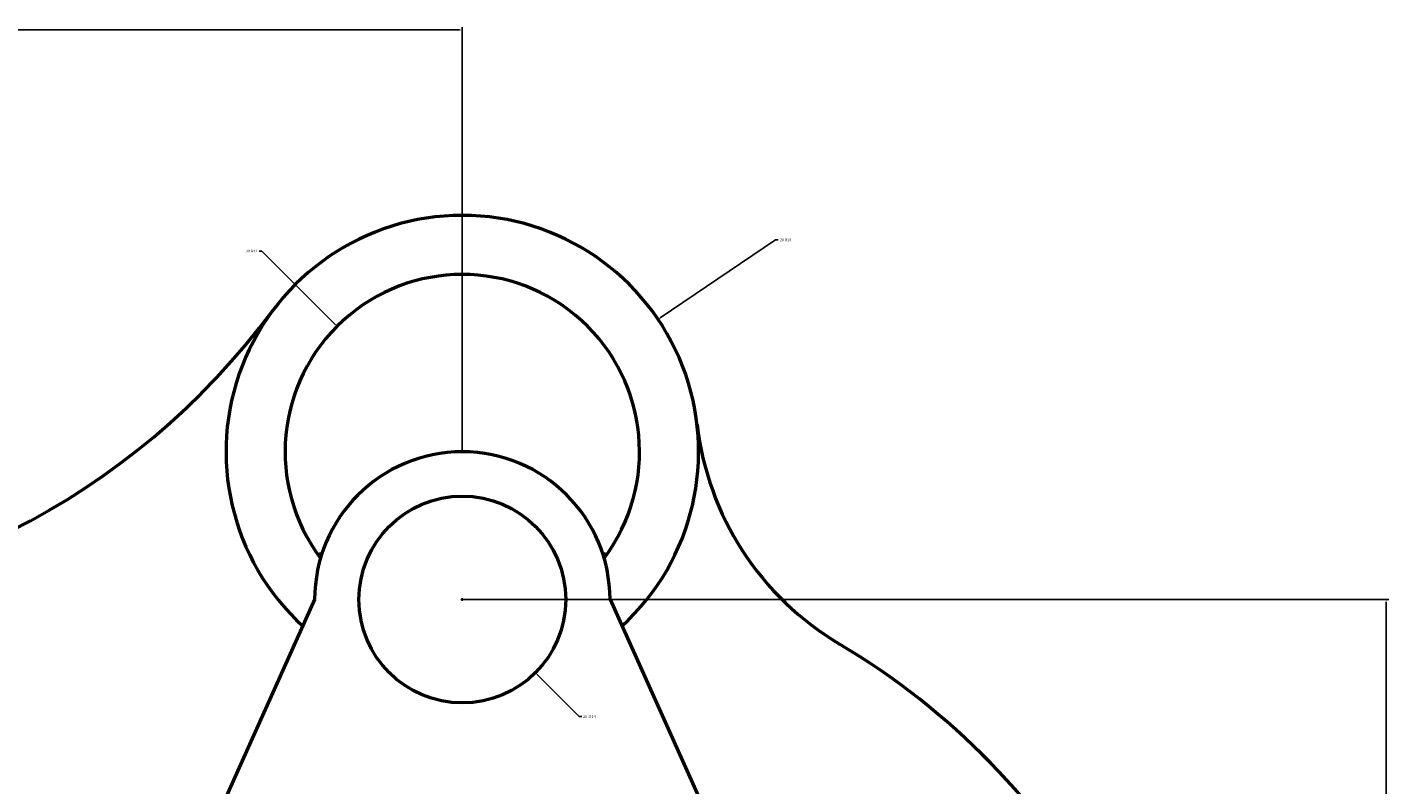
# Model space of a CAD drawing. Units: inches. Extents: x -307 to -76, y 16 to 196.
# Tile 7 of 7: x -168 to -76, y 134 to 186. Entities that reach past the tile are written whole.
import ezdxf

# ---------------------------------------------------------------- set-up
doc = ezdxf.new("R2010")
doc.units = ezdxf.units.IN
doc.header["$MEASUREMENT"] = 0
for name, color, linetype, lineweight in [('M-DIMS', 2, 'Continuous', 18), ('M-OUTL', 7, 'Continuous', 50), ('M-OUTL-LINK', 7, 'Continuous', 50)]:
    doc.layers.add(name, color=color, linetype=linetype, lineweight=lineweight)
doc.styles.get("Standard").update_dxf_attribs({"font": 'arial.ttf'})
doc.dimstyles.get("Standard").update_dxf_attribs({"dimtxt": 0.18, "dimasz": 0.18, "dimexe": 0.18, "dimexo": 0.0625, "dimgap": 0.09, "dimtad": 0, "dimtih": 1, "dimtoh": 1, "dimdec": 4, "dimzin": 0, "dimdsep": 46, "dimtxsty": 'Standard', "dimcen": 0.09, "dimadec": 0, "dimazin": 0, "dimtfac": 1, "dimtdec": 4, "dimtofl": 0, "dimtmove": 0, "dimatfit": 3, "dimfxl": 1, "dimtolj": 1, "dimtzin": 0, "dimarcsym": 0})

# ---------------------------------------------------------------- blocks, each defined once
blk = doc.blocks.new('*D5')
at = {"layer": 'Defpoints', "color": 0, "transparency": 16777216}
for p in [(-138.39, 185.55), (-138.39, 157), (-203.39, 101)]:
    blk.add_point(p, dxfattribs=at)
at = {"layer": 'M-DIMS', "color": 0, "lineweight": -2, "transparency": 16777216}
for p, q in [((-203.39, 101.062), (-203.39, 185.73)), ((-203.21, 185.55), (-171.11, 185.55)), ((-138.57, 185.55), (-170.67, 185.55)), ((-138.39, 157.062), (-138.39, 185.73))]:
    blk.add_line(p, q, dxfattribs=at)
at = {"layer": 'M-DIMS', "color": 0, "transparency": 16777216}
for points in [[(-203.21, 185.58), (-203.21, 185.52), (-203.39, 185.55)], [(-138.57, 185.58), (-138.57, 185.52), (-138.39, 185.55)]]:
    blk.add_solid(points, dxfattribs=at)
at = {"layer": 'M-DIMS', "color": 0, "transparency": 16777216, "insert": (-170.89, 185.55), "char_height": 0.18, "attachment_point": 5}
blk.add_mtext('\\A1;65', dxfattribs=at)
blk = doc.blocks.new('*D9')
at = {"layer": 'Defpoints', "color": 0, "transparency": 16777216}
for p in [(-138.39, 147), (-75.84, 147), (-138.39, 101)]:
    blk.add_point(p, dxfattribs=at)
at = {"layer": 'M-DIMS', "color": 0, "lineweight": -2, "transparency": 16777216}
for p, q in [((-138.327, 147), (-75.66, 147)), ((-75.84, 146.82), (-75.84, 124.182)), ((-75.84, 101.18), (-75.84, 123.818)), ((-138.327, 101), (-75.66, 101))]:
    blk.add_line(p, q, dxfattribs=at)
at = {"layer": 'M-DIMS', "color": 0, "transparency": 16777216}
for points in [[(-75.87, 146.82), (-75.81, 146.82), (-75.84, 147)], [(-75.87, 101.18), (-75.81, 101.18), (-75.84, 101)]]:
    blk.add_solid(points, dxfattribs=at)
at = {"layer": 'M-DIMS', "color": 0, "transparency": 16777216, "insert": (-75.84, 124), "char_height": 0.18, "attachment_point": 5}
blk.add_mtext('\\A1;46', dxfattribs=at)
blk = doc.blocks.new('*D15')
at = {"layer": 'Defpoints', "color": 0, "transparency": 16777216}
for p in [(-125.134, 165.96), (-138.39, 157)]:
    blk.add_point(p, dxfattribs=at)
at = {"layer": 'M-DIMS', "color": 0, "lineweight": -2, "transparency": 16777216}
for p, q in [((-117.18, 171.336), (-124.985, 166.061)), ((-117, 171.336), (-117.18, 171.336)), ((-138.48, 157), (-138.3, 157)), ((-138.39, 156.91), (-138.39, 157.09))]:
    blk.add_line(p, q, dxfattribs=at)
at = {"layer": 'M-DIMS', "color": 0, "transparency": 16777216}
blk.add_solid([(-125.002, 166.086), (-124.968, 166.036), (-125.134, 165.96)], dxfattribs=at)
at = {"layer": 'M-DIMS', "color": 0, "transparency": 16777216, "insert": (-116.5, 171.336), "char_height": 0.18, "attachment_point": 5}
blk.add_mtext('\\A1;2X R16', dxfattribs=at)
blk = doc.blocks.new('*D16')
at = {"layer": 'Defpoints', "color": 0, "transparency": 16777216}
for p in [(-146.875, 165.485), (-138.39, 157)]:
    blk.add_point(p, dxfattribs=at)
at = {"layer": 'M-DIMS', "color": 0, "lineweight": -2, "transparency": 16777216}
for p, q in [((-152.146, 170.576), (-151.966, 170.576)), ((-151.966, 170.576), (-147.002, 165.612)), ((-138.48, 157), (-138.3, 157)), ((-138.39, 156.91), (-138.39, 157.09))]:
    blk.add_line(p, q, dxfattribs=at)
at = {"layer": 'M-DIMS', "color": 0, "transparency": 16777216}
blk.add_solid([(-146.981, 165.634), (-147.024, 165.591), (-146.875, 165.485)], dxfattribs=at)
at = {"layer": 'M-DIMS', "color": 0, "transparency": 16777216, "insert": (-152.645, 170.576), "char_height": 0.18, "attachment_point": 5}
blk.add_mtext('\\A1;2X R12', dxfattribs=at)
blk = doc.blocks.new('*D18')
at = {"layer": 'Defpoints', "color": 0, "transparency": 16777216}
for p in [(-143.339, 151.95), (-133.44, 142.05)]:
    blk.add_point(p, dxfattribs=at)
at = {"layer": 'M-DIMS', "color": 0, "lineweight": -2, "transparency": 16777216}
for p, q in [((-138.48, 147), (-138.3, 147)), ((-138.39, 146.91), (-138.39, 147.09)), ((-130.47, 139.08), (-133.313, 141.923)), ((-130.29, 139.08), (-130.47, 139.08))]:
    blk.add_line(p, q, dxfattribs=at)
at = {"layer": 'M-DIMS', "color": 0, "transparency": 16777216}
blk.add_solid([(-133.292, 141.944), (-133.334, 141.902), (-133.44, 142.05)], dxfattribs=at)
at = {"layer": 'M-DIMS', "color": 0, "transparency": 16777216, "insert": (-129.784, 139.08), "char_height": 0.18, "attachment_point": 5}
blk.add_mtext('\\A1;2X ∅14', dxfattribs=at)

msp = doc.modelspace()

# ---------------------------------------------------------------- linework, layer by layer
at = {"layer": 'M-OUTL'}
for centre, radius, start, end in [((-138.39, 157), 16, 312.49719, 227.50281), ((-138.39, 157), 12, 323.1301, 216.8699), ((-191.39, 196.332), 50, 216.57954, 323.42046), ((-102.633, 161.179), 20, 186.66543, 239.28223), ((-138.39, 101), 50, 100.96633, 101.27083), ((-138.39, 101), 50, 78.72917, 79.03367), ((-138.39, 101), 50, 300.71777, 59.28223)]:
    msp.add_arc(centre, radius, start, end, dxfattribs=at)
at = {"layer": 'M-OUTL-LINK'}
for p, q in [((-148.39, 147), (-163.922, 112.493)), ((-128.39, 147), (-112.857, 112.493))]:
    msp.add_line(p, q, dxfattribs=at)
msp.add_circle((-138.39, 147), 7, dxfattribs=at)
msp.add_arc((-138.39, 147), 10, 0, 180, dxfattribs=at)

# ---------------------------------------------------------------- dimensions: what is measured, and where the dimension line sits
at = {"layer": 'M-DIMS'}
dim = msp.add_linear_dim(base=(-138.39, 185.55), p1=(-203.39, 101), p2=(-138.39, 157), dimstyle='Standard', override={"dimdec": 0, "dimlfac": 1, "dimrnd": 0, "dimzin": 0, "dimdsep": 46, "dimlunit": 2}, dxfattribs=at)
dim.commit()
dim.dimension.update_dxf_attribs({"geometry": '*D5', "text_midpoint": (-170.89, 185.55)})
for mpoint, picture, middle in [((-125.134, 165.96), '*D15', (-116.5, 171.336)), ((-146.875, 165.485), '*D16', (-152.645, 170.576))]:
    dim = msp.add_radius_dim(center=(-138.39, 157), mpoint=mpoint, text='2X <>', dimstyle='Standard', override={"dimdec": 0, "dimlfac": 1, "dimrnd": 0, "dimzin": 0, "dimdsep": 46, "dimlunit": 2}, dxfattribs=at)
    dim.commit()
    dim.dimension.update_dxf_attribs({"geometry": picture, "text_midpoint": middle, "dimtype": 164})
dim = msp.add_diameter_dim_2p(p1=(-143.339, 151.95), p2=(-133.44, 142.05), text='2X <>', dimstyle='Standard', override={"dimdec": 0, "dimlfac": 1, "dimrnd": 0, "dimzin": 0, "dimdsep": 46, "dimlunit": 2}, dxfattribs=at)
dim.commit()
dim.dimension.update_dxf_attribs({"geometry": '*D18', "text_midpoint": (-129.784, 139.08), "dimtype": 163})
dim = msp.add_linear_dim(base=(-75.84, 147), p1=(-138.39, 101), p2=(-138.39, 147), angle=90, dimstyle='Standard', override={"dimdec": 0, "dimlfac": 1, "dimrnd": 0, "dimzin": 0, "dimdsep": 46, "dimlunit": 2}, dxfattribs=at)
dim.commit()
dim.dimension.update_dxf_attribs({"geometry": '*D9', "text_midpoint": (-75.84, 124)})

doc.saveas('drawing.dxf')
